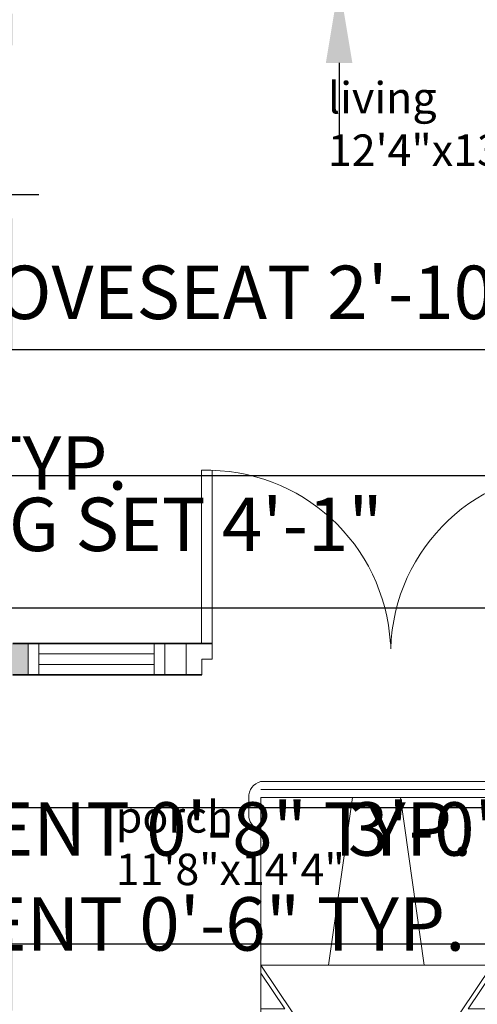
# Model space of a CAD drawing. Units: inches. Extents: x 19 to 15718, y 7 to 930.
# Tile 9 of 11: x 15415 to 15502, y 458 to 646. Entities that reach past the tile are written whole.
import ezdxf

# ---------------------------------------------------------------- set-up
doc = ezdxf.new("R2010")
doc.units = ezdxf.units.IN
doc.header["$MEASUREMENT"] = 0
for name, color, linetype, lineweight in [('A-ANNO-DIMS', 2, 'Continuous', 18), ('A-AREA-IDEN', 7, 'Continuous', 18), ('A-DOOR', 4, 'Continuous', 20), ('A-GLAZ', 4, 'Continuous', 18), ('A-WALL', 7, 'Continuous', 35), ('C-PKNG-VEHC', 8, 'Continuous', 13)]:
    doc.layers.add(name, color=color, linetype=linetype, lineweight=lineweight)
doc.layers.add('A-WALL-PATT', color=18, linetype='Continuous', lineweight=13, true_color=0x000000)
doc.styles.add('Annotative', font='arial.ttf')
doc.styles.get("Standard").update_dxf_attribs({"font": 'arial.ttf'})
doc.dimstyles.get("Standard").update_dxf_attribs({"dimtxt": 10.18, "dimasz": 15.18, "dimexe": 0.18, "dimexo": 0.0625, "dimgap": 0.09, "dimtad": 0, "dimtih": 1, "dimtoh": 1, "dimdec": 0, "dimzin": 0, "dimdsep": 46, "dimlunit": 3, "dimtxsty": 'Standard', "dimcen": 0.09, "dimadec": 0, "dimazin": 0, "dimtfac": 1, "dimtdec": 0, "dimtofl": 0, "dimtmove": 0, "dimatfit": 3, "dimfxl": 1, "dimtolj": 1, "dimtzin": 0, "dimarcsym": 0})

# ---------------------------------------------------------------- blocks, each defined once
blk = doc.blocks.new('*U14')
for p, q in [((5.44, 42.31), (12.12, 42.31)), ((189.69, 42.31), (183.01, 42.31)), ((0.1, -0.41), (0.1, 38.35)), ((2.77, -0.41), (2.77, 38.31)), ((5.44, -0.41), (5.44, 38.24)), ((5.45, 38.31), (16.12, 38.31)), ((16.12, 38.31), (180.34, 38.31)), ((61.52, -0.41), (61.52, 38.31)), ((61.52, 38.31), (77.54, 27.62)), ((64.19, 38.31), (76.2, 30.29)), ((76.2, 30.29), (76.2, 38.31)), ((78.87, 38.31), (78.87, 28.96)), ((106.91, 28.96), (106.91, 38.31)), ((109.58, 27.62), (109.58, 38.31)), ((112.25, 38.31), (112.25, 28.96)), ((140.29, 28.96), (140.29, 38.31)), ((141.62, 27.62), (149.64, 38.31)), ((149.64, -0.41), (149.64, 38.31)), ((189.69, 38.31), (179.01, 38.31)), ((189.69, -0.41), (189.69, 38.24)), ((192.36, -0.41), (192.36, 38.31)), ((195.03, -0.41), (195.03, 38.35)), ((77.54, 27.62), (141.62, 27.62)), ((77.54, -0.41), (77.54, 27.62)), ((78.87, 28.96), (106.91, 28.96)), ((112.25, 28.96), (140.29, 28.96)), ((141.62, -0.41), (141.62, 27.62)), ((5.44, 7.6), (61.52, 15.61)), ((0.1, -0.42), (0.1, -39.18)), ((2.77, -0.41), (2.77, -39.13)), ((5.44, -0.42), (5.44, -39.07)), ((61.52, -0.41), (61.52, -39.13)), ((77.54, -0.41), (77.54, -28.45)), ((141.62, -0.41), (141.62, -28.45)), ((149.64, -0.41), (149.64, -39.13)), ((189.69, -0.42), (189.69, -39.07)), ((192.36, -0.41), (192.36, -39.13)), ((195.03, -0.42), (195.03, -39.18)), ((5.44, -8.42), (61.52, -16.43)), ((61.52, -39.13), (77.54, -28.45)), ((77.54, -28.45), (141.62, -28.45)), ((109.58, -28.45), (109.58, -39.13)), ((141.62, -28.45), (149.64, -39.13)), ((64.19, -39.13), (76.2, -31.12)), ((76.2, -31.12), (76.2, -39.13)), ((78.87, -39.13), (78.87, -29.79)), ((78.87, -29.79), (106.91, -29.79)), ((106.91, -29.79), (106.91, -39.13)), ((112.25, -29.79), (140.29, -29.79)), ((112.25, -39.13), (112.25, -29.79)), ((140.29, -29.79), (140.29, -39.13)), ((5.45, -39.13), (16.12, -39.13)), ((16.12, -39.13), (180.34, -39.13)), ((189.69, -39.13), (179.01, -39.13)), ((5.44, -43.14), (12.12, -43.14)), ((189.69, -43.14), (183.01, -43.14))]:
    blk.add_line(p, q)
for centre, radius, start, end in [((5.06, 37.26), 5.06, 85.6455, 168.0943), ((11.45, 37.64), 4.72, 8.1301, 81.87), ((183.68, 37.64), 4.72, 98.13, 171.8699), ((190.07, 37.26), 5.06, 11.9057, 94.3545), ((5.06, -38.09), 5.06, 191.9057, 274.3545), ((11.45, -38.46), 4.72, 278.13, 351.8699), ((183.68, -38.46), 4.72, 188.1301, 261.87), ((190.07, -38.09), 5.06, 265.6455, 348.0943)]:
    blk.add_arc(centre, radius, start, end)
blk = doc.blocks.new('DOOR-ENTRY-LEAF-36IN')
for p, q in [((0, 6), (0, 39)), ((2, 3), (2, 39)), ((0, 3), (0, 0)), ((2, 3), (0, 3))]:
    blk.add_line(p, q)
blk.add_arc((1, 4), 35.01, 1.6366, 91.6366)
blk = doc.blocks.new('*D46')
at = {"layer": 'A-ANNO-DIMS', "color": 0, "lineweight": -2, "transparency": 16777216}
for p, q in [((15343.07, 612.73), (15327.89, 612.73)), ((15358.25, 608.29), (15358.25, 612.91)), ((15388.25, 608.29), (15388.25, 612.91)), ((15403.43, 612.73), (15418.61, 612.73))]:
    blk.add_line(p, q, dxfattribs=at)
at = {"layer": 'A-ANNO-DIMS', "color": 0, "transparency": 16777216}
for points in [[(15343.07, 615.26), (15343.07, 610.2), (15358.25, 612.73)], [(15403.43, 615.26), (15403.43, 610.2), (15388.25, 612.73)]]:
    blk.add_solid(points, dxfattribs=at)
at = {"layer": 'Defpoints', "color": 0, "transparency": 16777216}
for p in [(15358.25, 612.73), (15358.25, 608.23), (15388.25, 608.23)]:
    blk.add_point(p, dxfattribs=at)
at = {"layer": 'A-ANNO-DIMS', "color": 0, "transparency": 16777216, "insert": (15257.09, 612.73), "char_height": 10.18, "attachment_point": 5}
blk.add_mtext('\\A1;BASIN TOP 2\'-6" TYP.', dxfattribs=at)
blk = doc.blocks.new('*D62')
at = {"layer": 'A-ANNO-DIMS', "color": 0, "lineweight": -2, "transparency": 16777216}
for p, q in [((15269.83, 473.76), (15254.65, 473.76)), ((15285.01, 474.6), (15285.01, 473.58)), ((15291.01, 474.6), (15291.01, 473.58)), ((15306.19, 473.76), (15321.37, 473.76))]:
    blk.add_line(p, q, dxfattribs=at)
at = {"layer": 'A-ANNO-DIMS', "color": 0, "transparency": 16777216}
for points in [[(15269.83, 476.29), (15269.83, 471.23), (15285.01, 473.76)], [(15306.19, 476.29), (15306.19, 471.23), (15291.01, 473.76)]]:
    blk.add_solid(points, dxfattribs=at)
at = {"layer": 'Defpoints', "color": 0, "transparency": 16777216}
for p in [(15285.01, 474.66), (15291.01, 474.66), (15291.01, 473.76)]:
    blk.add_point(p, dxfattribs=at)
at = {"layer": 'A-ANNO-DIMS', "color": 0, "transparency": 16777216, "insert": (15413.32, 473.76), "char_height": 10.18, "attachment_point": 5}
blk.add_mtext('\\A1;SMALL ELEMENT 0\'-6" TYP.', dxfattribs=at)
blk = doc.blocks.new('*D64')
at = {"layer": 'A-ANNO-DIMS', "color": 0, "lineweight": -2, "transparency": 16777216}
for p, q in [((15268.83, 491.86), (15253.65, 491.86)), ((15284.01, 490.72), (15284.01, 492.04)), ((15292.01, 490.72), (15292.01, 492.04)), ((15307.19, 491.86), (15322.37, 491.86))]:
    blk.add_line(p, q, dxfattribs=at)
at = {"layer": 'A-ANNO-DIMS', "color": 0, "transparency": 16777216}
for points in [[(15268.83, 494.39), (15268.83, 489.33), (15284.01, 491.86)], [(15307.19, 494.39), (15307.19, 489.33), (15292.01, 491.86)]]:
    blk.add_solid(points, dxfattribs=at)
at = {"layer": 'Defpoints', "color": 0, "transparency": 16777216}
for p in [(15292.01, 491.86), (15284.01, 490.66), (15292.01, 490.66)]:
    blk.add_point(p, dxfattribs=at)
at = {"layer": 'A-ANNO-DIMS', "color": 0, "transparency": 16777216, "insert": (15414.9, 491.86), "char_height": 10.18, "attachment_point": 5}
blk.add_mtext('\\A1;LARGE ELEMENT 0\'-8" TYP.', dxfattribs=at)
blk = doc.blocks.new('*D67')
at = {"layer": 'A-ANNO-DIMS', "color": 0, "lineweight": -2, "transparency": 16777216}
for p, q in [((15329.76, 563.64), (15329.76, 561.42)), ((15343.51, 563.64), (15343.51, 561.42)), ((15314.58, 561.6), (15299.4, 561.6)), ((15358.69, 561.6), (15373.87, 561.6))]:
    blk.add_line(p, q, dxfattribs=at)
at = {"layer": 'A-ANNO-DIMS', "color": 0, "transparency": 16777216}
for points in [[(15314.58, 564.13), (15314.58, 559.07), (15329.76, 561.6)], [(15358.69, 564.13), (15358.69, 559.07), (15343.51, 561.6)]]:
    blk.add_solid(points, dxfattribs=at)
at = {"layer": 'Defpoints', "color": 0, "transparency": 16777216}
for p in [(15329.76, 563.7), (15343.51, 563.7), (15343.51, 561.6)]:
    blk.add_point(p, dxfattribs=at)
at = {"layer": 'A-ANNO-DIMS', "color": 0, "transparency": 16777216, "insert": (15404.51, 561.6), "char_height": 10.18, "attachment_point": 5}
blk.add_mtext('\\A1;1\'-2" TYP.', dxfattribs=at)
blk = doc.blocks.new('*D68')
at = {"layer": 'A-ANNO-DIMS', "color": 0, "lineweight": -2, "transparency": 16777216}
for p, q in [((15309.3, 542.58), (15309.3, 550.07)), ((15324.48, 549.89), (15343.27, 549.89)), ((15358.45, 542.58), (15358.45, 550.07)), ((15358.45, 549.89), (15373.63, 549.89))]:
    blk.add_line(p, q, dxfattribs=at)
at = {"layer": 'A-ANNO-DIMS', "color": 0, "transparency": 16777216}
for points in [[(15324.48, 552.42), (15324.48, 547.36), (15309.3, 549.89)], [(15343.27, 552.42), (15343.27, 547.36), (15358.45, 549.89)]]:
    blk.add_solid(points, dxfattribs=at)
at = {"layer": 'Defpoints', "color": 0, "transparency": 16777216}
for p in [(15358.45, 549.89), (15309.3, 542.52), (15358.45, 542.52)]:
    blk.add_point(p, dxfattribs=at)
at = {"layer": 'A-ANNO-DIMS', "color": 0, "transparency": 16777216, "insert": (15429.66, 549.89), "char_height": 10.18, "attachment_point": 5}
blk.add_mtext('\\A1;DINING SET 4\'-1"', dxfattribs=at)
blk = doc.blocks.new('*D71')
at = {"layer": 'A-ANNO-DIMS', "color": 0, "lineweight": -2, "transparency": 16777216}
for p, q in [((15475.84, 687.74), (15475.84, 702.92)), ((15482.5, 672.56), (15475.66, 672.56)), ((15482.5, 652.99), (15475.66, 652.99)), ((15475.84, 637.81), (15475.84, 622.63))]:
    blk.add_line(p, q, dxfattribs=at)
at = {"layer": 'A-ANNO-DIMS', "color": 0, "transparency": 16777216}
for points in [[(15473.31, 687.74), (15478.37, 687.74), (15475.84, 672.56)], [(15473.31, 637.81), (15478.37, 637.81), (15475.84, 652.99)]]:
    blk.add_solid(points, dxfattribs=at)
at = {"layer": 'Defpoints', "color": 0, "transparency": 16777216}
for p in [(15475.84, 672.56), (15482.56, 672.56), (15482.56, 652.99)]:
    blk.add_point(p, dxfattribs=at)
at = {"layer": 'A-ANNO-DIMS', "color": 0, "transparency": 16777216, "insert": (15475.84, 662.77), "char_height": 10.18, "attachment_point": 5}
blk.add_mtext('\\A1;1\'-7 1/2"', dxfattribs=at)
blk = doc.blocks.new('*D72')
at = {"layer": 'A-ANNO-DIMS', "color": 0, "lineweight": -2, "transparency": 16777216}
for p, q in [((15548.36, 643.79), (15553.66, 643.79)), ((15553.48, 628.61), (15553.48, 624.46)), ((15548.36, 609.28), (15553.66, 609.28)), ((15553.48, 609.28), (15553.48, 594.1)), ((15553.48, 594.1), (15538.3, 594.1))]:
    blk.add_line(p, q, dxfattribs=at)
at = {"layer": 'A-ANNO-DIMS', "color": 0, "transparency": 16777216}
for points in [[(15550.95, 628.61), (15556.01, 628.61), (15553.48, 643.79)], [(15550.95, 624.46), (15556.01, 624.46), (15553.48, 609.28)]]:
    blk.add_solid(points, dxfattribs=at)
at = {"layer": 'Defpoints', "color": 0, "transparency": 16777216}
for p in [(15548.3, 643.79), (15548.3, 609.28), (15553.48, 609.28)]:
    blk.add_point(p, dxfattribs=at)
at = {"layer": 'A-ANNO-DIMS', "color": 0, "transparency": 16777216, "insert": (15469.57, 594.1), "char_height": 10.18, "attachment_point": 5}
blk.add_mtext('\\A1;LOVESEAT 2\'-10 1/2"', dxfattribs=at)
blk = doc.blocks.new('*D73')
at = {"layer": 'A-ANNO-DIMS', "color": 0, "lineweight": -2, "transparency": 16777216}
for p, q in [((15527.21, 643.85), (15527.21, 649.15)), ((15548.3, 643.85), (15548.3, 649.15)), ((15512.03, 648.97), (15496.85, 648.97)), ((15563.48, 648.97), (15578.66, 648.97))]:
    blk.add_line(p, q, dxfattribs=at)
at = {"layer": 'A-ANNO-DIMS', "color": 0, "transparency": 16777216}
for points in [[(15512.03, 651.5), (15512.03, 646.44), (15527.21, 648.97)], [(15563.48, 651.5), (15563.48, 646.44), (15548.3, 648.97)]]:
    blk.add_solid(points, dxfattribs=at)
at = {"layer": 'Defpoints', "color": 0, "transparency": 16777216}
for p in [(15548.3, 648.97), (15527.21, 643.79), (15548.3, 643.79)]:
    blk.add_point(p, dxfattribs=at)
at = {"layer": 'A-ANNO-DIMS', "color": 0, "transparency": 16777216, "insert": (15591.8, 648.97), "char_height": 10.18, "attachment_point": 5}
blk.add_mtext('\\A1;1\'-9"', dxfattribs=at)
blk = doc.blocks.new('*D79')
at = {"layer": 'A-ANNO-DIMS', "color": 0, "lineweight": -2, "transparency": 16777216}
for p, q in [((15602.03, 534), (15602.03, 549.18)), ((15602.03, 549.18), (15617.21, 549.18)), ((15082.89, 534), (15602.21, 534)), ((15602.03, 511.14), (15602.03, 518.82)), ((15082.89, 495.96), (15602.21, 495.96))]:
    blk.add_line(p, q, dxfattribs=at)
at = {"layer": 'A-ANNO-DIMS', "color": 0, "transparency": 16777216}
for points in [[(15599.5, 518.82), (15604.56, 518.82), (15602.03, 534)], [(15599.5, 511.14), (15604.56, 511.14), (15602.03, 495.96)]]:
    blk.add_solid(points, dxfattribs=at)
at = {"layer": 'Defpoints', "color": 0, "transparency": 16777216}
for p in [(15082.83, 534), (15602.03, 534), (15082.83, 495.96)]:
    blk.add_point(p, dxfattribs=at)
at = {"layer": 'A-ANNO-DIMS', "color": 0, "transparency": 16777216, "insert": (15630.83, 549.18), "char_height": 10.18, "attachment_point": 5}
blk.add_mtext('\\A1;3\'-2"', dxfattribs=at)
blk = doc.blocks.new('*D80')
at = {"layer": 'A-ANNO-DIMS', "color": 0, "lineweight": -2, "transparency": 16777216}
for p, q in [((15602.030581, 511.142303), (15602.030581, 526.322303)), ((15181.899116, 495.962303), (15602.210581, 495.962303)), ((15181.899116, 469.995573), (15602.210581, 469.995573)), ((15602.030581, 454.815573), (15602.030581, 439.635573))]:
    blk.add_line(p, q, dxfattribs=at)
at = {"layer": 'A-ANNO-DIMS', "color": 0, "transparency": 16777216}
for points in [[(15599.500581, 511.142303), (15604.560581, 511.142303), (15602.030581, 495.962303)], [(15599.500581, 454.815573), (15604.560581, 454.815573), (15602.030581, 469.995573)]]:
    blk.add_solid(points, dxfattribs=at)
at = {"layer": 'Defpoints', "color": 0, "transparency": 16777216}
for p in [(15181.836616, 495.962303), (15602.030581, 495.962303), (15181.836616, 469.995573)]:
    blk.add_point(p, dxfattribs=at)
at = {"layer": 'A-ANNO-DIMS', "color": 0, "transparency": 16777216, "insert": (15602.030581, 482.978938), "char_height": 10.18, "attachment_point": 5}
blk.add_mtext('\\A1;2\'-2"', dxfattribs=at)
blk = doc.blocks.new('*D82')
at = {"layer": 'A-ANNO-DIMS', "color": 0, "lineweight": -2, "transparency": 16777216}
for p, q in [((15602.030581, 598.383955), (15602.030581, 613.563955)), ((15377.073779, 583.203955), (15602.210581, 583.203955)), ((15377.073779, 559.203955), (15602.210581, 559.203955)), ((15602.030581, 544.023955), (15602.030581, 528.843955))]:
    blk.add_line(p, q, dxfattribs=at)
at = {"layer": 'A-ANNO-DIMS', "color": 0, "transparency": 16777216}
for points in [[(15599.500581, 598.383955), (15604.560581, 598.383955), (15602.030581, 583.203955)], [(15599.500581, 544.023955), (15604.560581, 544.023955), (15602.030581, 559.203955)]]:
    blk.add_solid(points, dxfattribs=at)
at = {"layer": 'Defpoints', "color": 0, "transparency": 16777216}
for p in [(15377.011279, 583.203955), (15602.030581, 583.203955), (15377.011279, 559.203955)]:
    blk.add_point(p, dxfattribs=at)
at = {"layer": 'A-ANNO-DIMS', "color": 0, "transparency": 16777216, "insert": (15602.030581, 571.203955), "char_height": 10.18, "attachment_point": 5}
blk.add_mtext('\\A1;2\'-0"', dxfattribs=at)
blk = doc.blocks.new('*D85')
at = {"layer": 'A-ANNO-DIMS', "color": 0, "lineweight": -2, "transparency": 16777216}
for p, q in [((15521.68, 527.14), (15521.68, 491.67)), ((15557.68, 527.14), (15557.68, 491.67)), ((15521.68, 491.85), (15506.5, 491.85)), ((15542.5, 491.85), (15536.86, 491.85))]:
    blk.add_line(p, q, dxfattribs=at)
at = {"layer": 'A-ANNO-DIMS', "color": 0, "transparency": 16777216}
for points in [[(15536.86, 494.38), (15536.86, 489.32), (15521.68, 491.85)], [(15542.5, 494.38), (15542.5, 489.32), (15557.68, 491.85)]]:
    blk.add_solid(points, dxfattribs=at)
at = {"layer": 'Defpoints', "color": 0, "transparency": 16777216}
for p in [(15521.68, 527.2), (15557.68, 527.2), (15521.68, 491.85)]:
    blk.add_point(p, dxfattribs=at)
at = {"layer": 'A-ANNO-DIMS', "color": 0, "transparency": 16777216, "insert": (15492.88, 491.85), "char_height": 10.18, "attachment_point": 5}
blk.add_mtext('\\A1;3\'-0"', dxfattribs=at)

msp = doc.modelspace()

# ---------------------------------------------------------------- hatches: boundary and pattern name
at = {"layer": 'A-WALL-PATT'}
h = msp.add_hatch(color=256, dxfattribs=at)
h.dxf.hatch_style = 1
h.paths.add_polyline_path([(15566.68, 830.2), (15266.68, 830.2), (15266.68, 629.2), (15275.68, 629.2), (15275.68, 641.2), (15301.68, 641.2), (15301.68, 589.2), (15275.68, 589.2), (15275.68, 601.2), (15266.68, 601.2), (15266.68, 350.2), (15275.68, 350.2), (15275.68, 359.2), (15275.68, 457.2), (15413.68, 457.2), (15413.68, 471.04), (15407.68, 471.04), (15407.68, 463.2), (15275.68, 463.2), (15275.68, 583.59), (15276.07, 583.2), (15276.65, 583.2), (15277.42, 583.97), (15276.36, 585.03), (15279.54, 588.22), (15280.6, 587.16), (15281.66, 588.22), (15282.72, 587.16), (15283.78, 588.22), (15284.85, 587.16), (15285.91, 588.22), (15286.97, 587.16), (15288.03, 588.22), (15289.09, 587.16), (15290.15, 588.22), (15291.21, 587.16), (15292.27, 588.22), (15293.33, 587.16), (15294.39, 588.22), (15295.45, 587.16), (15296.51, 588.22), (15297.57, 587.16), (15298.63, 588.22), (15299.69, 587.16), (15300.76, 588.22), (15301.82, 587.16), (15302.88, 588.22), (15303.94, 587.16), (15305, 588.22), (15306.06, 587.16), (15307.68, 588.78), (15307.68, 641.2), (15407.68, 641.2), (15413.68, 641.2), (15413.68, 647.2), (15407.68, 647.2), (15275.68, 647.2), (15275.68, 767.2), (15336.68, 767.2), (15336.68, 773.2), (15275.68, 773.2), (15275.68, 821.2), (15375.68, 821.2), (15381.68, 821.2), (15407.68, 821.2), (15413.68, 821.2), (15557.68, 821.2), (15557.68, 697.2), (15452.68, 697.2), (15452.68, 696.2, -0.014283), (15452.68, 694.2), (15452.68, 691.2), (15557.68, 691.2), (15557.68, 527.2), (15557.68, 521.2), (15557.68, 359.2), (15557.68, 350.2), (15566.68, 350.2)])
h.paths.add_polyline_path([(15416.63, 527.2), (15413.68, 527.2), (15407.68, 527.2), (15407.68, 521.04), (15413.68, 521.04), (15413.68, 521.2), (15416.63, 521.2)], flags=17)
h.paths.add_polyline_path([(15432.13, 393.97), (15308.13, 393.97), (15308.13, 425.59), (15299.13, 425.59), (15299.13, 384.97), (15432.13, 384.97)], flags=17)
h.paths.add_polyline_path([(15308.13, 457.2), (15299.13, 457.2), (15299.13, 425.59), (15308.13, 425.59)], flags=17)
h.paths.add_polyline_path([(15425.57, 359.2), (15275.68, 359.2), (15275.68, 350.2), (15425.57, 350.2)], flags=17)
h.paths.add_polyline_path([(15413.68, 797.2), (15407.68, 797.2), (15407.68, 773.2), (15381.68, 773.2), (15381.68, 797.2), (15375.68, 797.2), (15375.68, 773.2), (15375.68, 767.2), (15407.68, 767.2), (15407.68, 686.2), (15408.68, 686.2, -0.014283), (15410.68, 686.2), (15413.68, 686.2), (15413.68, 691.2), (15413.68, 697.2)], flags=17)
h.paths.add_polyline_path([(15413.68, 608.2), (15410.68, 608.2, -0.017236), (15408.68, 608.2), (15407.68, 608.2), (15407.68, 589.2), (15388.16, 589.2, -0.313626), (15386.75, 588.23), (15381.37, 588.23), (15380.3, 587.16), (15381.37, 586.1), (15380.3, 585.03), (15382.14, 583.2), (15407.68, 583.2), (15413.68, 583.2)], flags=17)

# ---------------------------------------------------------------- linework, layer by layer
at = {"layer": 'A-DOOR'}
for p, q in [((15449.65, 527.2), (15449.65, 560.2)), ((15451.65, 524.2), (15451.65, 560.2)), ((15446.68, 521.2), (15446.68, 527.2)), ((15485.61, 527.2), (15485.72, 527.2)), ((15485.68, 526.2), (15485.68, 527.2)), ((15449.68, 521.2), (15449.68, 524.2)), ((15451.65, 524.2), (15449.68, 524.2))]:
    msp.add_line(p, q, dxfattribs=at)
msp.add_arc((15450.65, 525.2), 35.01, 3.2745, 91.6366, dxfattribs=at)
at = {"layer": 'A-GLAZ'}
for p, q in [((15416.63, 527.2), (15416.63, 521.2)), ((15418.63, 527.2), (15418.63, 521.2)), ((15440.63, 527.2), (15440.63, 521.2)), ((15442.63, 527.2), (15442.63, 521.2)), ((15418.63, 525.2), (15440.63, 525.2)), ((15418.63, 523.2), (15440.63, 523.2))]:
    msp.add_line(p, q, dxfattribs=at)
at = {"layer": 'A-WALL'}
for p, q in [((15413.68, 527.2), (15451.65, 527.2)), ((15413.68, 521.2), (15449.68, 521.2))]:
    msp.add_line(p, q, dxfattribs=at)

# ---------------------------------------------------------------- block references
at = {"layer": 'A-DOOR', "extrusion": (0, 0, -1), "zscale": -1}
msp.add_blockref('DOOR-ENTRY-LEAF-36IN', (-15521.68, 521.2), dxfattribs=at)
at = {"layer": 'C-PKNG-VEHC', "xscale": 0.5691226359303588, "yscale": 0.5691226359303588, "zscale": 0.5691226359303588, "rotation": 270}
msp.add_blockref('*U14', (15483.19, 500.93), dxfattribs=at)

# ---------------------------------------------------------------- texts
at = {"layer": 'A-AREA-IDEN', "char_height": 6, "width": 68.1983, "attachment_point": 1, "style": 'Annotative'}
for s, insert in [('living\\P12\'4"x13\'8"', (15473.71, 634.19)), ('porch\\P11\'8"x14\'4"', (15433.29, 497.15))]:
    msp.add_mtext(s, dxfattribs=dict(at, insert=insert))

# ---------------------------------------------------------------- dimensions: what is measured, and where the dimension line sits
at = {"layer": 'A-ANNO-DIMS'}
for base, p1, p2, angle, picture, middle in [((15475.84, 672.56), (15482.56, 652.99), (15482.56, 672.56), 90, '*D71', (15475.84, 662.77)), ((15602.03, 583.2), (15377.01, 559.2), (15377.01, 583.2), 90, '*D82', (15602.03, 571.2)), ((15602.03, 534), (15082.83, 495.96), (15082.83, 534), 90, '*D79', (15630.83, 549.18)), ((15521.68, 491.85), (15557.68, 527.2), (15521.68, 527.2), 180, '*D85', (15492.88, 491.85)), ((15602.03, 495.96), (15181.84, 470), (15181.84, 495.96), 90, '*D80', (15602.03, 482.98))]:
    dim = msp.add_linear_dim(base=base, p1=p1, p2=p2, angle=angle, dimstyle='Standard', override={"dimdec": 1, "dimlfac": 1, "dimrnd": 0, "dimzin": 1, "dimdsep": 46, "dimlunit": 4, "dimfrac": 2}, dxfattribs=at)
    dim.commit()
    dim.dimension.update_dxf_attribs({"geometry": picture, "text_midpoint": middle})
dim = msp.add_linear_dim(base=(15548.3, 648.97), p1=(15527.21, 643.79), p2=(15548.3, 643.79), dimstyle='Standard', override={"dimdec": 1, "dimlfac": 1, "dimrnd": 0, "dimzin": 1, "dimdsep": 46, "dimlunit": 4, "dimfrac": 2}, dxfattribs=at)
dim.commit()
dim.dimension.update_dxf_attribs({"geometry": '*D73', "text_midpoint": (15591.8, 648.97)})
for base, p1, p2, angle, text, picture, middle in [((15358.25, 612.73), (15388.25, 608.23), (15358.25, 608.23), 180, 'BASIN TOP <> TYP.', '*D46', (15257.09, 612.73)), ((15553.48, 609.28), (15548.3, 643.79), (15548.3, 609.28), 270, 'LOVESEAT <>', '*D72', (15469.57, 594.1))]:
    dim = msp.add_linear_dim(base=base, p1=p1, p2=p2, angle=angle, text=text, dimstyle='Standard', override={"dimdec": 1, "dimlfac": 1, "dimrnd": 0, "dimzin": 1, "dimdsep": 46, "dimlunit": 4, "dimfrac": 2}, dxfattribs=at)
    dim.commit()
    dim.dimension.update_dxf_attribs({"geometry": picture, "text_midpoint": middle})
for base, p1, p2, text, picture, middle in [((15343.51127927, 561.60395495), (15329.76127927, 563.70395495), (15343.51127927, 563.70395495), '<> TYP.', '*D67', (15404.50822333, 561.60395495)), ((15358.4492, 549.8921), (15309.3028, 542.5201), (15358.4492, 542.5201), 'DINING SET <>', '*D68', (15429.664, 549.8921)), ((15292.01, 491.86), (15284.01, 490.66), (15292.01, 490.66), 'LARGE ELEMENT <> TYP.', '*D64', (15414.9, 491.86)), ((15291.01, 473.76), (15285.01, 474.66), (15291.01, 474.66), 'SMALL ELEMENT <> TYP.', '*D62', (15413.32, 473.76))]:
    dim = msp.add_linear_dim(base=base, p1=p1, p2=p2, text=text, dimstyle='Standard', override={"dimdec": 1, "dimlfac": 1, "dimrnd": 0, "dimzin": 1, "dimdsep": 46, "dimlunit": 4, "dimfrac": 2}, dxfattribs=at)
    dim.commit()
    dim.dimension.update_dxf_attribs({"geometry": picture, "text_midpoint": middle})

doc.saveas('drawing.dxf')
